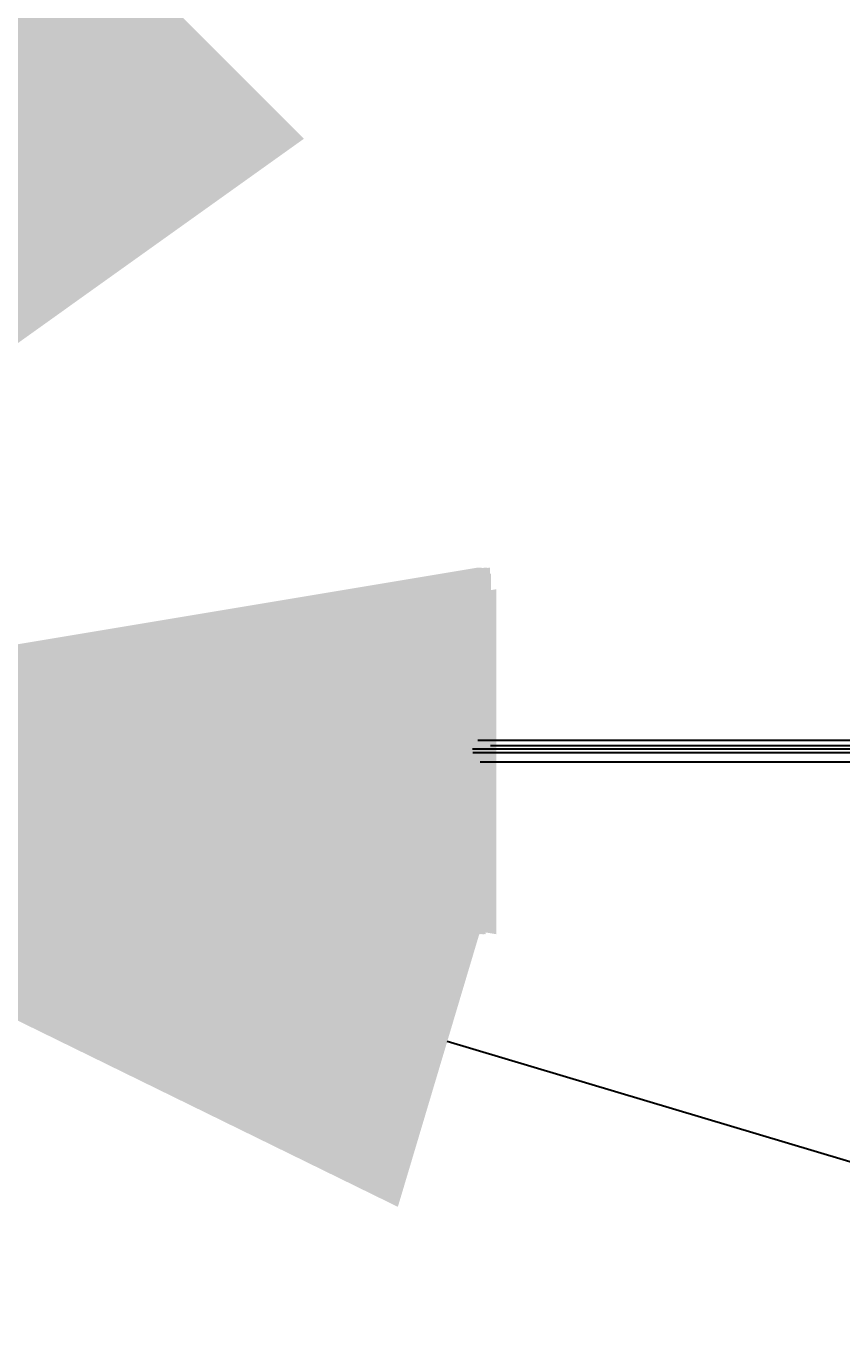
# Model space of a CAD drawing. Units: millimetres. Extents: x -22994 to 29398, y -19990 to 20176.
# Tile 133 of 135: x 5745 to 13629, y -5571 to 7102. Entities that reach past the tile are written whole.
import ezdxf

# ---------------------------------------------------------------- set-up
doc = ezdxf.new("R2010")
doc.units = ezdxf.units.MM
doc.header["$MEASUREMENT"] = 0
doc.layers.add('M-DIMS', color=2, linetype='Continuous', lineweight=18)
doc.styles.get("Standard").update_dxf_attribs({"font": 'arial.ttf'})
doc.dimstyles.get("Standard").update_dxf_attribs({"dimtxt": 0.18, "dimasz": 10000, "dimexe": 0.18, "dimexo": 0.0625, "dimgap": 0.09, "dimtad": 0, "dimtih": 1, "dimtoh": 1, "dimdec": 0, "dimzin": 0, "dimdsep": 46, "dimtxsty": 'Standard', "dimcen": 0.09, "dimadec": 0, "dimazin": 0, "dimtfac": 1, "dimtdec": 0, "dimtofl": 0, "dimtmove": 0, "dimatfit": 3, "dimfxl": 1, "dimtolj": 1, "dimtzin": 0, "dimlwd": 30, "dimarcsym": 0})

# ---------------------------------------------------------------- blocks, each defined once
blk = doc.blocks.new('*D2')
at = {"layer": 'Defpoints', "color": 0, "transparency": 16777216}
for p in [(7, 10), (291, 10), (291, -5)]:
    blk.add_point(p, dxfattribs=at)
at = {"layer": 'M-DIMS', "color": 0, "lineweight": -2, "transparency": 16777216}
for p, q in [((7, 10), (7, -5)), ((291, 10), (291, -5))]:
    blk.add_line(p, q, dxfattribs=at)
at = {"layer": 'M-DIMS', "color": 0, "lineweight": 30, "transparency": 16777216}
for p, q in [((-9993, -5), (-19993, -5)), ((10291, -5), (20291, -5))]:
    blk.add_line(p, q, dxfattribs=at)
at = {"layer": 'M-DIMS', "color": 0, "transparency": 16777216}
for points in [[(-9993, 1662), (-9993, -1672), (7, -5)], [(10291, 1662), (10291, -1672), (291, -5)]]:
    blk.add_solid(points, dxfattribs=at)
at = {"layer": 'M-DIMS', "color": 0, "transparency": 16777216, "insert": (149, -5), "char_height": 0.18, "attachment_point": 5}
blk.add_mtext('\\A1;284.2', dxfattribs=at)
blk = doc.blocks.new('*D3')
at = {"layer": 'Defpoints', "color": 0, "transparency": 16777216}
for p in [(96, 128), (110, 204), (110, 176)]:
    blk.add_point(p, dxfattribs=at)
at = {"layer": 'M-DIMS', "color": 0, "lineweight": 30, "transparency": 16777216}
for p, q in [((-9904, 204), (-19904, 204)), ((10110, 204), (20110, 204))]:
    blk.add_line(p, q, dxfattribs=at)
at = {"layer": 'M-DIMS', "color": 0, "lineweight": -2, "transparency": 16777216}
for p, q in [((96, 128), (96, 204)), ((110, 176), (110, 204))]:
    blk.add_line(p, q, dxfattribs=at)
at = {"layer": 'M-DIMS', "color": 0, "transparency": 16777216}
for points in [[(-9904, 1871), (-9904, -1463), (96, 204)], [(10110, 1871), (10110, -1463), (110, 204)]]:
    blk.add_solid(points, dxfattribs=at)
at = {"layer": 'M-DIMS', "color": 0, "transparency": 16777216, "insert": (103, 204), "char_height": 0.18, "attachment_point": 5}
blk.add_mtext('\\A1;14.432', dxfattribs=at)
blk = doc.blocks.new('*D4')
at = {"layer": 'Defpoints', "color": 0, "transparency": 16777216}
for p in [(110, 176), (116, 204), (116, 176)]:
    blk.add_point(p, dxfattribs=at)
at = {"layer": 'M-DIMS', "color": 0, "lineweight": 30, "transparency": 16777216}
for p, q in [((-9890, 204), (-19890, 204)), ((10116, 204), (20116, 204))]:
    blk.add_line(p, q, dxfattribs=at)
at = {"layer": 'M-DIMS', "color": 0, "lineweight": -2, "transparency": 16777216}
for p, q in [((110, 176), (110, 204)), ((116, 176), (116, 204))]:
    blk.add_line(p, q, dxfattribs=at)
at = {"layer": 'M-DIMS', "color": 0, "transparency": 16777216}
for points in [[(-9890, 1871), (-9890, -1463), (110, 204)], [(10116, 1871), (10116, -1463), (116, 204)]]:
    blk.add_solid(points, dxfattribs=at)
at = {"layer": 'M-DIMS', "color": 0, "transparency": 16777216, "insert": (113, 204), "char_height": 0.18, "attachment_point": 5}
blk.add_mtext('\\A1;6', dxfattribs=at)
blk = doc.blocks.new('*D5')
at = {"layer": 'Defpoints', "color": 0, "transparency": 16777216}
for p in [(116, 176), (181, 204), (181, 176)]:
    blk.add_point(p, dxfattribs=at)
at = {"layer": 'M-DIMS', "color": 0, "lineweight": 30, "transparency": 16777216}
for p, q in [((-9884, 204), (-19884, 204)), ((10181, 204), (20181, 204))]:
    blk.add_line(p, q, dxfattribs=at)
at = {"layer": 'M-DIMS', "color": 0, "lineweight": -2, "transparency": 16777216}
for p, q in [((116, 176), (116, 204)), ((181, 176), (181, 204))]:
    blk.add_line(p, q, dxfattribs=at)
at = {"layer": 'M-DIMS', "color": 0, "transparency": 16777216}
for points in [[(-9884, 1871), (-9884, -1463), (116, 204)], [(10181, 1871), (10181, -1463), (181, 204)]]:
    blk.add_solid(points, dxfattribs=at)
at = {"layer": 'M-DIMS', "color": 0, "transparency": 16777216, "insert": (149, 204), "char_height": 0.18, "attachment_point": 5}
blk.add_mtext('\\A1;65', dxfattribs=at)
blk = doc.blocks.new('*D6')
at = {"layer": 'Defpoints', "color": 0, "transparency": 16777216}
for p in [(181, 176), (187, 204), (187, 176)]:
    blk.add_point(p, dxfattribs=at)
at = {"layer": 'M-DIMS', "color": 0, "lineweight": 30, "transparency": 16777216}
for p, q in [((-9819, 204), (-19819, 204)), ((10187, 204), (20187, 204))]:
    blk.add_line(p, q, dxfattribs=at)
at = {"layer": 'M-DIMS', "color": 0, "lineweight": -2, "transparency": 16777216}
for p, q in [((181, 176), (181, 204)), ((187, 176), (187, 204))]:
    blk.add_line(p, q, dxfattribs=at)
at = {"layer": 'M-DIMS', "color": 0, "transparency": 16777216}
for points in [[(-9819, 1871), (-9819, -1463), (181, 204)], [(10187, 1871), (10187, -1463), (187, 204)]]:
    blk.add_solid(points, dxfattribs=at)
at = {"layer": 'M-DIMS', "color": 0, "transparency": 16777216, "insert": (184, 204), "char_height": 0.18, "attachment_point": 5}
blk.add_mtext('\\A1;6', dxfattribs=at)
blk = doc.blocks.new('*D7')
at = {"layer": 'Defpoints', "color": 0, "transparency": 16777216}
for p in [(187, 176), (202, 204), (202, 128)]:
    blk.add_point(p, dxfattribs=at)
at = {"layer": 'M-DIMS', "color": 0, "lineweight": 30, "transparency": 16777216}
for p, q in [((-9813, 204), (-19813, 204)), ((10202, 204), (20202, 204))]:
    blk.add_line(p, q, dxfattribs=at)
at = {"layer": 'M-DIMS', "color": 0, "lineweight": -2, "transparency": 16777216}
for p, q in [((187, 176), (187, 204)), ((202, 128), (202, 204))]:
    blk.add_line(p, q, dxfattribs=at)
at = {"layer": 'M-DIMS', "color": 0, "transparency": 16777216}
for points in [[(-9813, 1871), (-9813, -1463), (187, 204)], [(10202, 1871), (10202, -1463), (202, 204)]]:
    blk.add_solid(points, dxfattribs=at)
at = {"layer": 'M-DIMS', "color": 0, "transparency": 16777216, "insert": (194, 204), "char_height": 0.18, "attachment_point": 5}
blk.add_mtext('\\A1;14.432', dxfattribs=at)
blk = doc.blocks.new('*D8')
at = {"layer": 'Defpoints', "color": 0, "transparency": 16777216}
for p in [(202, 128), (228, 204), (228, 147)]:
    blk.add_point(p, dxfattribs=at)
at = {"layer": 'M-DIMS', "color": 0, "lineweight": 30, "transparency": 16777216}
for p, q in [((-9798, 204), (-19798, 204)), ((10228, 204), (20228, 204))]:
    blk.add_line(p, q, dxfattribs=at)
at = {"layer": 'M-DIMS', "color": 0, "lineweight": -2, "transparency": 16777216}
for p, q in [((202, 128), (202, 204)), ((228, 147), (228, 204))]:
    blk.add_line(p, q, dxfattribs=at)
at = {"layer": 'M-DIMS', "color": 0, "transparency": 16777216}
for points in [[(-9798, 1871), (-9798, -1463), (202, 204)], [(10228, 1871), (10228, -1463), (228, 204)]]:
    blk.add_solid(points, dxfattribs=at)
at = {"layer": 'M-DIMS', "color": 0, "transparency": 16777216, "insert": (215, 204), "char_height": 0.18, "attachment_point": 5}
blk.add_mtext('\\A1;25.95', dxfattribs=at)
blk = doc.blocks.new('*D10')
at = {"layer": 'Defpoints', "color": 0, "transparency": 16777216}
for p in [(126, 136), (133, 136), (133, -5)]:
    blk.add_point(p, dxfattribs=at)
at = {"layer": 'M-DIMS', "color": 0, "lineweight": -2, "transparency": 16777216}
for p, q in [((126, 136), (126, -5)), ((133, 136), (133, -5))]:
    blk.add_line(p, q, dxfattribs=at)
at = {"layer": 'M-DIMS', "color": 0, "lineweight": 30, "transparency": 16777216}
for p, q in [((-9874, -5), (-19874, -5)), ((10133, -5), (20133, -5))]:
    blk.add_line(p, q, dxfattribs=at)
at = {"layer": 'M-DIMS', "color": 0, "transparency": 16777216}
for points in [[(-9874, 1662), (-9874, -1672), (126, -5)], [(10133, 1662), (10133, -1672), (133, -5)]]:
    blk.add_solid(points, dxfattribs=at)
at = {"layer": 'M-DIMS', "color": 0, "transparency": 16777216, "insert": (129, -5), "char_height": 0.18, "attachment_point": 5}
blk.add_mtext('\\A1;7.696', dxfattribs=at)
blk = doc.blocks.new('*D11')
at = {"layer": 'Defpoints', "color": 0, "transparency": 16777216}
for p in [(133, 136), (136, 136), (136, -5)]:
    blk.add_point(p, dxfattribs=at)
at = {"layer": 'M-DIMS', "color": 0, "lineweight": -2, "transparency": 16777216}
for p, q in [((133, 136), (133, -5)), ((136, 136), (136, -5))]:
    blk.add_line(p, q, dxfattribs=at)
at = {"layer": 'M-DIMS', "color": 0, "lineweight": 30, "transparency": 16777216}
for p, q in [((-9867, -5), (-19867, -5)), ((10136, -5), (20136, -5))]:
    blk.add_line(p, q, dxfattribs=at)
at = {"layer": 'M-DIMS', "color": 0, "transparency": 16777216}
for points in [[(-9867, 1662), (-9867, -1672), (133, -5)], [(10136, 1662), (10136, -1672), (136, -5)]]:
    blk.add_solid(points, dxfattribs=at)
at = {"layer": 'M-DIMS', "color": 0, "transparency": 16777216, "insert": (134, -5), "char_height": 0.18, "attachment_point": 5}
blk.add_mtext('\\A1;2.304', dxfattribs=at)
blk = doc.blocks.new('*D12')
at = {"layer": 'Defpoints', "color": 0, "transparency": 16777216}
for p in [(136, 136), (146, 136), (146, -5)]:
    blk.add_point(p, dxfattribs=at)
at = {"layer": 'M-DIMS', "color": 0, "lineweight": -2, "transparency": 16777216}
for p, q in [((136, 136), (136, -5)), ((146, 136), (146, -5))]:
    blk.add_line(p, q, dxfattribs=at)
at = {"layer": 'M-DIMS', "color": 0, "lineweight": 30, "transparency": 16777216}
for p, q in [((-9864, -5), (-19864, -5)), ((10146, -5), (20146, -5))]:
    blk.add_line(p, q, dxfattribs=at)
at = {"layer": 'M-DIMS', "color": 0, "transparency": 16777216}
for points in [[(-9864, 1662), (-9864, -1672), (136, -5)], [(10146, 1662), (10146, -1672), (146, -5)]]:
    blk.add_solid(points, dxfattribs=at)
at = {"layer": 'M-DIMS', "color": 0, "transparency": 16777216, "insert": (141, -5), "char_height": 0.18, "attachment_point": 5}
blk.add_mtext('\\A1;10', dxfattribs=at)
blk = doc.blocks.new('*D13')
at = {"layer": 'Defpoints', "color": 0, "transparency": 16777216}
for p in [(146, 136), (156, 136), (156, -5)]:
    blk.add_point(p, dxfattribs=at)
at = {"layer": 'M-DIMS', "color": 0, "lineweight": -2, "transparency": 16777216}
for p, q in [((146, 136), (146, -5)), ((156, 136), (156, -5))]:
    blk.add_line(p, q, dxfattribs=at)
at = {"layer": 'M-DIMS', "color": 0, "lineweight": 30, "transparency": 16777216}
for p, q in [((-9854, -5), (-19854, -5)), ((10156, -5), (20156, -5))]:
    blk.add_line(p, q, dxfattribs=at)
at = {"layer": 'M-DIMS', "color": 0, "transparency": 16777216}
for points in [[(-9854, 1662), (-9854, -1672), (146, -5)], [(10156, 1662), (10156, -1672), (156, -5)]]:
    blk.add_solid(points, dxfattribs=at)
at = {"layer": 'M-DIMS', "color": 0, "transparency": 16777216, "insert": (151, -5), "char_height": 0.18, "attachment_point": 5}
blk.add_mtext('\\A1;10', dxfattribs=at)
blk = doc.blocks.new('*D14')
at = {"layer": 'Defpoints', "color": 0, "transparency": 16777216}
for p in [(156, 136), (166, 136), (166, -5)]:
    blk.add_point(p, dxfattribs=at)
at = {"layer": 'M-DIMS', "color": 0, "lineweight": -2, "transparency": 16777216}
for p, q in [((156, 136), (156, -5)), ((166, 136), (166, -5))]:
    blk.add_line(p, q, dxfattribs=at)
at = {"layer": 'M-DIMS', "color": 0, "lineweight": 30, "transparency": 16777216}
for p, q in [((-9844, -5), (-19844, -5)), ((10166, -5), (20166, -5))]:
    blk.add_line(p, q, dxfattribs=at)
at = {"layer": 'M-DIMS', "color": 0, "transparency": 16777216}
for points in [[(-9844, 1662), (-9844, -1672), (156, -5)], [(10166, 1662), (10166, -1672), (166, -5)]]:
    blk.add_solid(points, dxfattribs=at)
at = {"layer": 'M-DIMS', "color": 0, "transparency": 16777216, "insert": (161, -5), "char_height": 0.18, "attachment_point": 5}
blk.add_mtext('\\A1;10', dxfattribs=at)
blk = doc.blocks.new('*D16')
at = {"layer": 'Defpoints', "color": 0, "transparency": 16777216}
for p in [(120, 204), (110, 48), (120, 48)]:
    blk.add_point(p, dxfattribs=at)
at = {"layer": 'M-DIMS', "color": 0, "lineweight": 30, "transparency": 16777216}
for p, q in [((-9890, 204), (-19890, 204)), ((10120, 204), (20120, 204))]:
    blk.add_line(p, q, dxfattribs=at)
at = {"layer": 'M-DIMS', "color": 0, "lineweight": -2, "transparency": 16777216}
for p, q in [((110, 48), (110, 204)), ((120, 48), (120, 204))]:
    blk.add_line(p, q, dxfattribs=at)
at = {"layer": 'M-DIMS', "color": 0, "transparency": 16777216}
for points in [[(-9890, 1871), (-9890, -1463), (110, 204)], [(10120, 1871), (10120, -1463), (120, 204)]]:
    blk.add_solid(points, dxfattribs=at)
at = {"layer": 'M-DIMS', "color": 0, "transparency": 16777216, "insert": (115, 204), "char_height": 0.18, "attachment_point": 5}
blk.add_mtext('\\A1;9.704', dxfattribs=at)
blk = doc.blocks.new('*D17')
at = {"layer": 'Defpoints', "color": 0, "transparency": 16777216}
for p in [(126, 204), (120, 48), (126, 48)]:
    blk.add_point(p, dxfattribs=at)
at = {"layer": 'M-DIMS', "color": 0, "lineweight": 30, "transparency": 16777216}
for p, q in [((-9880, 204), (-19880, 204)), ((10126, 204), (20126, 204))]:
    blk.add_line(p, q, dxfattribs=at)
at = {"layer": 'M-DIMS', "color": 0, "lineweight": -2, "transparency": 16777216}
for p, q in [((120, 48), (120, 204)), ((126, 48), (126, 204))]:
    blk.add_line(p, q, dxfattribs=at)
at = {"layer": 'M-DIMS', "color": 0, "transparency": 16777216}
for points in [[(-9880, 1871), (-9880, -1463), (120, 204)], [(10126, 1871), (10126, -1463), (126, 204)]]:
    blk.add_solid(points, dxfattribs=at)
at = {"layer": 'M-DIMS', "color": 0, "transparency": 16777216, "insert": (123, 204), "char_height": 0.18, "attachment_point": 5}
blk.add_mtext('\\A1;6', dxfattribs=at)
blk = doc.blocks.new('*D18')
at = {"layer": 'Defpoints', "color": 0, "transparency": 16777216}
for p in [(132, 204), (126, 48), (132, 48)]:
    blk.add_point(p, dxfattribs=at)
at = {"layer": 'M-DIMS', "color": 0, "lineweight": 30, "transparency": 16777216}
for p, q in [((-9874, 204), (-19874, 204)), ((10132, 204), (20132, 204))]:
    blk.add_line(p, q, dxfattribs=at)
at = {"layer": 'M-DIMS', "color": 0, "lineweight": -2, "transparency": 16777216}
for p, q in [((126, 48), (126, 204)), ((132, 48), (132, 204))]:
    blk.add_line(p, q, dxfattribs=at)
at = {"layer": 'M-DIMS', "color": 0, "transparency": 16777216}
for points in [[(-9874, 1871), (-9874, -1463), (126, 204)], [(10132, 1871), (10132, -1463), (132, 204)]]:
    blk.add_solid(points, dxfattribs=at)
at = {"layer": 'M-DIMS', "color": 0, "transparency": 16777216, "insert": (129, 204), "char_height": 0.18, "attachment_point": 5}
blk.add_mtext('\\A1;6', dxfattribs=at)
blk = doc.blocks.new('*D19')
at = {"layer": 'Defpoints', "color": 0, "transparency": 16777216}
for p in [(138, 204), (132, 48), (138, 48)]:
    blk.add_point(p, dxfattribs=at)
at = {"layer": 'M-DIMS', "color": 0, "lineweight": 30, "transparency": 16777216}
for p, q in [((-9868, 204), (-19868, 204)), ((10138, 204), (20138, 204))]:
    blk.add_line(p, q, dxfattribs=at)
at = {"layer": 'M-DIMS', "color": 0, "lineweight": -2, "transparency": 16777216}
for p, q in [((132, 48), (132, 204)), ((138, 48), (138, 204))]:
    blk.add_line(p, q, dxfattribs=at)
at = {"layer": 'M-DIMS', "color": 0, "transparency": 16777216}
for points in [[(-9868, 1871), (-9868, -1463), (132, 204)], [(10138, 1871), (10138, -1463), (138, 204)]]:
    blk.add_solid(points, dxfattribs=at)
at = {"layer": 'M-DIMS', "color": 0, "transparency": 16777216, "insert": (135, 204), "char_height": 0.18, "attachment_point": 5}
blk.add_mtext('\\A1;6', dxfattribs=at)
blk = doc.blocks.new('*D20')
at = {"layer": 'Defpoints', "color": 0, "transparency": 16777216}
for p in [(144, 204), (138, 48), (144, 48)]:
    blk.add_point(p, dxfattribs=at)
at = {"layer": 'M-DIMS', "color": 0, "lineweight": 30, "transparency": 16777216}
for p, q in [((-9862, 204), (-19862, 204)), ((10144, 204), (20144, 204))]:
    blk.add_line(p, q, dxfattribs=at)
at = {"layer": 'M-DIMS', "color": 0, "lineweight": -2, "transparency": 16777216}
for p, q in [((138, 48), (138, 204)), ((144, 48), (144, 204))]:
    blk.add_line(p, q, dxfattribs=at)
at = {"layer": 'M-DIMS', "color": 0, "transparency": 16777216}
for points in [[(-9862, 1871), (-9862, -1463), (138, 204)], [(10144, 1871), (10144, -1463), (144, 204)]]:
    blk.add_solid(points, dxfattribs=at)
at = {"layer": 'M-DIMS', "color": 0, "transparency": 16777216, "insert": (141, 204), "char_height": 0.18, "attachment_point": 5}
blk.add_mtext('\\A1;6', dxfattribs=at)
blk = doc.blocks.new('*D21')
at = {"layer": 'Defpoints', "color": 0, "transparency": 16777216}
for p in [(149, 204), (144, 48), (149, 48)]:
    blk.add_point(p, dxfattribs=at)
at = {"layer": 'M-DIMS', "color": 0, "lineweight": 30, "transparency": 16777216}
for p, q in [((-9856, 204), (-19856, 204)), ((10149, 204), (20149, 204))]:
    blk.add_line(p, q, dxfattribs=at)
at = {"layer": 'M-DIMS', "color": 0, "lineweight": -2, "transparency": 16777216}
for p, q in [((144, 48), (144, 204)), ((149, 48), (149, 204))]:
    blk.add_line(p, q, dxfattribs=at)
at = {"layer": 'M-DIMS', "color": 0, "transparency": 16777216}
for points in [[(-9856, 1871), (-9856, -1463), (144, 204)], [(10149, 1871), (10149, -1463), (149, 204)]]:
    blk.add_solid(points, dxfattribs=at)
at = {"layer": 'M-DIMS', "color": 0, "transparency": 16777216, "insert": (147, 204), "char_height": 0.18, "attachment_point": 5}
blk.add_mtext('\\A1;4.945', dxfattribs=at)
blk = doc.blocks.new('*D22')
at = {"layer": 'Defpoints', "color": 0, "transparency": 16777216}
for p in [(149, 31), (155, 31), (155, -5)]:
    blk.add_point(p, dxfattribs=at)
at = {"layer": 'M-DIMS', "color": 0, "lineweight": -2, "transparency": 16777216}
for p, q in [((149, 31), (149, -5)), ((155, 31), (155, -5))]:
    blk.add_line(p, q, dxfattribs=at)
at = {"layer": 'M-DIMS', "color": 0, "lineweight": 30, "transparency": 16777216}
for p, q in [((-9851, -5), (-19851, -5)), ((10155, -5), (20155, -5))]:
    blk.add_line(p, q, dxfattribs=at)
at = {"layer": 'M-DIMS', "color": 0, "transparency": 16777216}
for points in [[(-9851, 1662), (-9851, -1672), (149, -5)], [(10155, 1662), (10155, -1672), (155, -5)]]:
    blk.add_solid(points, dxfattribs=at)
at = {"layer": 'M-DIMS', "color": 0, "transparency": 16777216, "insert": (152, -5), "char_height": 0.18, "attachment_point": 5}
blk.add_mtext('\\A1;6', dxfattribs=at)
blk = doc.blocks.new('*D23')
at = {"layer": 'Defpoints', "color": 0, "transparency": 16777216}
for p in [(155, 31), (161, 31), (161, -5)]:
    blk.add_point(p, dxfattribs=at)
at = {"layer": 'M-DIMS', "color": 0, "lineweight": -2, "transparency": 16777216}
for p, q in [((155, 31), (155, -5)), ((161, 31), (161, -5))]:
    blk.add_line(p, q, dxfattribs=at)
at = {"layer": 'M-DIMS', "color": 0, "lineweight": 30, "transparency": 16777216}
for p, q in [((-9845, -5), (-19845, -5)), ((10161, -5), (20161, -5))]:
    blk.add_line(p, q, dxfattribs=at)
at = {"layer": 'M-DIMS', "color": 0, "transparency": 16777216}
for points in [[(-9845, 1662), (-9845, -1672), (155, -5)], [(10161, 1662), (10161, -1672), (161, -5)]]:
    blk.add_solid(points, dxfattribs=at)
at = {"layer": 'M-DIMS', "color": 0, "transparency": 16777216, "insert": (158, -5), "char_height": 0.18, "attachment_point": 5}
blk.add_mtext('\\A1;6', dxfattribs=at)
blk = doc.blocks.new('*D24')
at = {"layer": 'Defpoints', "color": 0, "transparency": 16777216}
for p in [(161, 31), (166, 31), (166, -5)]:
    blk.add_point(p, dxfattribs=at)
at = {"layer": 'M-DIMS', "color": 0, "lineweight": -2, "transparency": 16777216}
for p, q in [((161, 31), (161, -5)), ((166, 31), (166, -5))]:
    blk.add_line(p, q, dxfattribs=at)
at = {"layer": 'M-DIMS', "color": 0, "lineweight": 30, "transparency": 16777216}
for p, q in [((-9839, -5), (-19839, -5)), ((10166, -5), (20166, -5))]:
    blk.add_line(p, q, dxfattribs=at)
at = {"layer": 'M-DIMS', "color": 0, "transparency": 16777216}
for points in [[(-9839, 1662), (-9839, -1672), (161, -5)], [(10166, 1662), (10166, -1672), (166, -5)]]:
    blk.add_solid(points, dxfattribs=at)
at = {"layer": 'M-DIMS', "color": 0, "transparency": 16777216, "insert": (164, -5), "char_height": 0.18, "attachment_point": 5}
blk.add_mtext('\\A1;5.323', dxfattribs=at)
blk = doc.blocks.new('*D25')
at = {"layer": 'Defpoints', "color": 0, "transparency": 16777216}
for p in [(166, 31), (172, 31), (172, -5)]:
    blk.add_point(p, dxfattribs=at)
at = {"layer": 'M-DIMS', "color": 0, "lineweight": -2, "transparency": 16777216}
for p, q in [((166, 31), (166, -5)), ((172, 31), (172, -5))]:
    blk.add_line(p, q, dxfattribs=at)
at = {"layer": 'M-DIMS', "color": 0, "lineweight": 30, "transparency": 16777216}
for p, q in [((-9834, -5), (-19834, -5)), ((10172, -5), (20172, -5))]:
    blk.add_line(p, q, dxfattribs=at)
at = {"layer": 'M-DIMS', "color": 0, "transparency": 16777216}
for points in [[(-9834, 1662), (-9834, -1672), (166, -5)], [(10172, 1662), (10172, -1672), (172, -5)]]:
    blk.add_solid(points, dxfattribs=at)
at = {"layer": 'M-DIMS', "color": 0, "transparency": 16777216, "insert": (169, -5), "char_height": 0.18, "attachment_point": 5}
blk.add_mtext('\\A1;6', dxfattribs=at)
blk = doc.blocks.new('*D26')
at = {"layer": 'Defpoints', "color": 0, "transparency": 16777216}
for p in [(172, 31), (178, 31), (178, -5)]:
    blk.add_point(p, dxfattribs=at)
at = {"layer": 'M-DIMS', "color": 0, "lineweight": -2, "transparency": 16777216}
for p, q in [((172, 31), (172, -5)), ((178, 31), (178, -5))]:
    blk.add_line(p, q, dxfattribs=at)
at = {"layer": 'M-DIMS', "color": 0, "lineweight": 30, "transparency": 16777216}
for p, q in [((-9828, -5), (-19828, -5)), ((10178, -5), (20178, -5))]:
    blk.add_line(p, q, dxfattribs=at)
at = {"layer": 'M-DIMS', "color": 0, "transparency": 16777216}
for points in [[(-9828, 1662), (-9828, -1672), (172, -5)], [(10178, 1662), (10178, -1672), (178, -5)]]:
    blk.add_solid(points, dxfattribs=at)
at = {"layer": 'M-DIMS', "color": 0, "transparency": 16777216, "insert": (175, -5), "char_height": 0.18, "attachment_point": 5}
blk.add_mtext('\\A1;6', dxfattribs=at)
blk = doc.blocks.new('*D27')
at = {"layer": 'Defpoints', "color": 0, "transparency": 16777216}
for p in [(178, 31), (188, 31), (188, -5)]:
    blk.add_point(p, dxfattribs=at)
at = {"layer": 'M-DIMS', "color": 0, "lineweight": -2, "transparency": 16777216}
for p, q in [((178, 31), (178, -5)), ((188, 31), (188, -5))]:
    blk.add_line(p, q, dxfattribs=at)
at = {"layer": 'M-DIMS', "color": 0, "lineweight": 30, "transparency": 16777216}
for p, q in [((-9822, -5), (-19822, -5)), ((10188, -5), (20188, -5))]:
    blk.add_line(p, q, dxfattribs=at)
at = {"layer": 'M-DIMS', "color": 0, "transparency": 16777216}
for points in [[(-9822, 1662), (-9822, -1672), (178, -5)], [(10188, 1662), (10188, -1672), (188, -5)]]:
    blk.add_solid(points, dxfattribs=at)
at = {"layer": 'M-DIMS', "color": 0, "transparency": 16777216, "insert": (183, -5), "char_height": 0.18, "attachment_point": 5}
blk.add_mtext('\\A1;9.679', dxfattribs=at)
blk = doc.blocks.new('*D29')
at = {"layer": 'Defpoints', "color": 0, "transparency": 16777216}
for p in [(37, 80), (64, 80)]:
    blk.add_point(p, dxfattribs=at)
at = {"layer": 'M-DIMS', "color": 0, "lineweight": -2, "transparency": 16777216}
for q in [(51, 80), (50, 80)]:
    blk.add_line((50, 80), q, dxfattribs=at)
at = {"layer": 'M-DIMS', "color": 0, "lineweight": 30, "transparency": 16777216}
blk.add_line((20064, 80), (10064, 80), dxfattribs=at)
at = {"layer": 'M-DIMS', "color": 0, "transparency": 16777216}
blk.add_solid([(10064, 1747), (10064, -1587), (64, 80)], dxfattribs=at)
at = {"layer": 'M-DIMS', "color": 0, "transparency": 16777216, "insert": (20065, 80), "char_height": 0.18, "attachment_point": 5}
blk.add_mtext('\\A1;∅27.23', dxfattribs=at)
blk = doc.blocks.new('*D30')
at = {"layer": 'Defpoints', "color": 0, "transparency": 16777216}
for p in [(216, 147), (239, 147)]:
    blk.add_point(p, dxfattribs=at)
at = {"layer": 'M-DIMS', "color": 0, "lineweight": -2, "transparency": 16777216}
blk.add_line((228, 147), (228, 147), dxfattribs=at)
blk.add_line((228, 147), (228, 147), dxfattribs=at)
at = {"layer": 'M-DIMS', "color": 0, "lineweight": 30, "transparency": 16777216}
blk.add_line((20239, 147), (10239, 147), dxfattribs=at)
at = {"layer": 'M-DIMS', "color": 0, "transparency": 16777216}
blk.add_solid([(10239, 1814), (10239, -1520), (239, 147)], dxfattribs=at)
at = {"layer": 'M-DIMS', "color": 0, "transparency": 16777216, "insert": (20240, 147), "char_height": 0.18, "attachment_point": 5}
blk.add_mtext('\\A1;∅22.667', dxfattribs=at)
blk = doc.blocks.new('*D31')
at = {"layer": 'Defpoints', "color": 0, "transparency": 16777216}
for p in [(223, 147), (232, 147)]:
    blk.add_point(p, dxfattribs=at)
at = {"layer": 'M-DIMS', "color": 0, "lineweight": -2, "transparency": 16777216}
blk.add_line((228, 147), (228, 147), dxfattribs=at)
blk.add_line((228, 147), (228, 147), dxfattribs=at)
at = {"layer": 'M-DIMS', "color": 0, "lineweight": 30, "transparency": 16777216}
blk.add_line((20232, 149), (10232, 148), dxfattribs=at)
at = {"layer": 'M-DIMS', "color": 0, "transparency": 16777216}
blk.add_solid([(10232, 1814), (10232, -1519), (232, 147)], dxfattribs=at)
at = {"layer": 'M-DIMS', "color": 0, "transparency": 16777216, "insert": (20233, 149), "char_height": 0.18, "attachment_point": 5}
blk.add_mtext('\\A1;∅8.969', dxfattribs=at)
blk = doc.blocks.new('*D33')
at = {"layer": 'Defpoints', "color": 0, "transparency": 16777216}
for p in [(230, 154), (233, 153)]:
    blk.add_point(p, dxfattribs=at)
at = {"layer": 'M-DIMS', "color": 0, "lineweight": -2, "transparency": 16777216}
for p in [(229, 154), (230, 154)]:
    blk.add_line(p, (230, 154), dxfattribs=at)
at = {"layer": 'M-DIMS', "color": 0, "lineweight": 30, "transparency": 16777216}
for p, q in [((19396, -5571), (9815, -2709)), ((29396, -5571), (19396, -5571))]:
    blk.add_line(p, q, dxfattribs=at)
at = {"layer": 'M-DIMS', "color": 0, "transparency": 16777216}
blk.add_solid([(10292, -1112), (9338, -4306), (233, 153)], dxfattribs=at)
at = {"layer": 'M-DIMS', "color": 0, "transparency": 16777216, "insert": (29397, -5571), "char_height": 0.18, "attachment_point": 5}
blk.add_mtext('\\A1;6X R3.586', dxfattribs=at)
blk = doc.blocks.new('*D34')
at = {"layer": 'Defpoints', "color": 0, "transparency": 16777216}
for p in [(177, 121), (179, 123)]:
    blk.add_point(p, dxfattribs=at)
at = {"layer": 'M-DIMS', "color": 0, "lineweight": 30, "transparency": 16777216}
for p, q in [((14322, 14263), (7251, 7193)), ((24322, 14263), (14322, 14263))]:
    blk.add_line(p, q, dxfattribs=at)
at = {"layer": 'M-DIMS', "color": 0, "lineweight": -2, "transparency": 16777216}
blk.add_line((177, 121), (177, 121), dxfattribs=at)
blk.add_line((177, 121), (177, 121), dxfattribs=at)
at = {"layer": 'M-DIMS', "color": 0, "transparency": 16777216}
blk.add_solid([(6072, 8372), (8429, 6014), (179, 123)], dxfattribs=at)
at = {"layer": 'M-DIMS', "color": 0, "transparency": 16777216, "insert": (24323, 14263), "char_height": 0.18, "attachment_point": 5}
blk.add_mtext('\\A1;6X R2.5', dxfattribs=at)
blk = doc.blocks.new('*D36')
at = {"layer": 'Defpoints', "color": 0, "transparency": 16777216}
for p in [(46, 31), (46, 27)]:
    blk.add_point(p, dxfattribs=at)
at = {"layer": 'M-DIMS', "color": 0, "lineweight": 30, "transparency": 16777216}
for p, q in [((57, 20031), (52, 10031)), ((10057, 20031), (57, 20031))]:
    blk.add_line(p, q, dxfattribs=at)
at = {"layer": 'M-DIMS', "color": 0, "lineweight": -2, "transparency": 16777216}
blk.add_line((46, 29), (46, 29), dxfattribs=at)
blk.add_line((46, 29), (46, 29), dxfattribs=at)
at = {"layer": 'M-DIMS', "color": 0, "transparency": 16777216}
blk.add_solid([(-1615, 10032), (1718, 10030), (46, 31)], dxfattribs=at)
at = {"layer": 'M-DIMS', "color": 0, "transparency": 16777216, "insert": (10058, 20031), "char_height": 0.18, "attachment_point": 5}
blk.add_mtext('\\A1;∅4.71', dxfattribs=at)
blk = doc.blocks.new('*D37')
at = {"layer": 'Defpoints', "color": 0, "transparency": 16777216}
for p in [(55, 119), (59, 119)]:
    blk.add_point(p, dxfattribs=at)
at = {"layer": 'M-DIMS', "color": 0, "lineweight": -2, "transparency": 16777216}
blk.add_line((57, 119), (57, 119), dxfattribs=at)
blk.add_line((57, 119), (57, 119), dxfattribs=at)
at = {"layer": 'M-DIMS', "color": 0, "lineweight": 30, "transparency": 16777216}
blk.add_line((20059, 116), (10059, 117), dxfattribs=at)
at = {"layer": 'M-DIMS', "color": 0, "transparency": 16777216}
blk.add_solid([(10060, 1784), (10059, -1549), (59, 119)], dxfattribs=at)
at = {"layer": 'M-DIMS', "color": 0, "transparency": 16777216, "insert": (20060, 116), "char_height": 0.18, "attachment_point": 5}
blk.add_mtext('\\A1;∅4.659', dxfattribs=at)

msp = doc.modelspace()

# ---------------------------------------------------------------- dimensions: what is measured, and where the dimension line sits
at = {"layer": 'M-DIMS'}
for p1, p2, override, picture, middle in [((46.3875, 26.5934), (46.39, 31.3035), {"dimdec": 2, "dimlfac": 1, "dimrnd": 0, "dimzin": 0, "dimdsep": 46, "dimlunit": 2}, '*D36', (10057.5542, 20031.3006)), ((216.3148, 146.7291), (238.9821, 146.73), {"dimdec": 3, "dimlfac": 1, "dimrnd": 0, "dimzin": 0, "dimdsep": 46, "dimlunit": 2}, '*D30', (20238.9821, 147.4959)), ((223.1641, 146.7291), (232.1328, 146.73), {"dimdec": 3, "dimlfac": 1, "dimrnd": 0, "dimzin": 0, "dimdsep": 46, "dimlunit": 2}, '*D31', (20232.1327, 148.6656))]:
    dim = msp.add_diameter_dim_2p(p1=p1, p2=p2, dimstyle='Standard', override=override, dxfattribs=at)
    dim.commit()
    dim.dimension.update_dxf_attribs({"geometry": picture, "text_midpoint": middle, "dimtype": 163})
for center, mpoint, override, picture, middle in [((176.8123, 121.1277), (178.5802, 122.8952), {"dimdec": 1, "dimlfac": 1, "dimrnd": 0, "dimzin": 0, "dimdsep": 46, "dimlunit": 2}, '*D34', (24322.9703, 14263.3108)), ((229.5613, 154.3773), (232.9972, 153.3509), {"dimdec": 3, "dimlfac": 1, "dimrnd": 0, "dimzin": 0, "dimdsep": 46, "dimlunit": 2}, '*D33', (29397.0125, -5570.8378))]:
    dim = msp.add_radius_dim(center=center, mpoint=mpoint, text='6X <>', dimstyle='Standard', override=override, dxfattribs=at)
    dim.commit()
    dim.dimension.update_dxf_attribs({"geometry": picture, "text_midpoint": middle})
for base, p1, p2, override, picture, middle in [((110.2647, 204.1654), (95.8327, 127.967), (110.2647, 176.3662), {"dimdec": 3, "dimlfac": 1, "dimrnd": 0, "dimzin": 0, "dimdsep": 46, "dimlunit": 2}, '*D3', (103.0487, 204.1654)), ((116.2647, 204.1654), (110.2647, 176.3662), (116.2647, 176.3662), {"dimdec": 0, "dimlfac": 1, "dimrnd": 0, "dimzin": 0, "dimdsep": 46, "dimlunit": 2}, '*D4', (113.2647, 204.1654)), ((120.1702, 204.1654), (110.4658, 48.0349), (120.1702, 48.0349), {"dimdec": 3, "dimlfac": 1, "dimrnd": 0, "dimzin": 0, "dimdsep": 46, "dimlunit": 2}, '*D16', (115.318, 204.1654)), ((181.2647, 204.1654), (116.2647, 176.3662), (181.2647, 176.3662), {"dimdec": 0, "dimlfac": 1, "dimrnd": 0, "dimzin": 0, "dimdsep": 46, "dimlunit": 2}, '*D5', (148.7647, 204.1654)), ((126.1702, 204.1654), (120.1702, 48.0349), (126.1702, 48.0349), {"dimdec": 0, "dimlfac": 1, "dimrnd": 0, "dimzin": 0, "dimdsep": 46, "dimlunit": 2}, '*D17', (123.1702, 204.1654)), ((132.1702, 204.1654), (126.1702, 48.0349), (132.1702, 48.0349), {"dimdec": 0, "dimlfac": 1, "dimrnd": 0, "dimzin": 0, "dimdsep": 46, "dimlunit": 2}, '*D18', (129.1702, 204.1654)), ((138.1702, 204.1654), (132.1702, 48.0349), (138.1702, 48.0349), {"dimdec": 0, "dimlfac": 1, "dimrnd": 0, "dimzin": 0, "dimdsep": 46, "dimlunit": 2}, '*D19', (135.1702, 204.1654)), ((144.1702, 204.1654), (138.1702, 48.0349), (144.1702, 48.0349), {"dimdec": 0, "dimlfac": 1, "dimrnd": 0, "dimzin": 0, "dimdsep": 46, "dimlunit": 2}, '*D20', (141.1702, 204.1654)), ((149.11567, 204.16539), (144.17023, 48.03494), (149.11567, 48.03494), {"dimdec": 3, "dimlfac": 1, "dimrnd": 0, "dimzin": 0, "dimdsep": 46, "dimlunit": 2}, '*D21', (146.64295, 204.16539)), ((187.2647, 204.1654), (181.2647, 176.3662), (187.2647, 176.3662), {"dimdec": 0, "dimlfac": 1, "dimrnd": 0, "dimzin": 0, "dimdsep": 46, "dimlunit": 2}, '*D6', (184.2647, 204.1654)), ((201.6967, 204.1654), (187.2647, 176.3662), (201.6967, 127.967), {"dimdec": 3, "dimlfac": 1, "dimrnd": 0, "dimzin": 0, "dimdsep": 46, "dimlunit": 2}, '*D7', (194.4807, 204.1654)), ((227.6485, 204.1654), (201.6967, 127.967), (227.6485, 146.7296), {"dimdec": 2, "dimlfac": 1, "dimrnd": 0, "dimzin": 0, "dimdsep": 46, "dimlunit": 2}, '*D8', (214.6726, 204.1654)), ((290.852, -5.0787), (6.6773, 10.2713), (290.852, 10.2713), {"dimdec": 1, "dimlfac": 1, "dimrnd": 0, "dimzin": 0, "dimdsep": 46, "dimlunit": 2}, '*D2', (148.7647, -5.0787)), ((133.3459, -5.0787), (125.6498, 136.0713), (133.3459, 136.0713), {"dimdec": 3, "dimlfac": 1, "dimrnd": 0, "dimzin": 0, "dimdsep": 46, "dimlunit": 2}, '*D10', (129.4978, -5.0787)), ((135.6498, -5.0787), (133.3459, 136.0713), (135.6498, 136.0713), {"dimdec": 3, "dimlfac": 1, "dimrnd": 0, "dimzin": 0, "dimdsep": 46, "dimlunit": 2}, '*D11', (134.4978, -5.0787)), ((145.6498, -5.0787), (135.6498, 136.0713), (145.6498, 136.0713), {"dimdec": 0, "dimlfac": 1, "dimrnd": 0, "dimzin": 0, "dimdsep": 46, "dimlunit": 2}, '*D12', (140.6498, -5.0787)), ((155.6498, -5.0787), (145.6498, 136.0713), (155.6498, 136.0713), {"dimdec": 0, "dimlfac": 1, "dimrnd": 0, "dimzin": 0, "dimdsep": 46, "dimlunit": 2}, '*D13', (150.6498, -5.0787)), ((155.1157, -5.0787), (149.1157, 30.9895), (155.1157, 30.9895), {"dimdec": 0, "dimlfac": 1, "dimrnd": 0, "dimzin": 0, "dimdsep": 46, "dimlunit": 2}, '*D22', (152.1157, -5.0787)), ((161.1157, -5.0787), (155.1157, 30.9895), (161.1157, 30.9895), {"dimdec": 0, "dimlfac": 1, "dimrnd": 0, "dimzin": 0, "dimdsep": 46, "dimlunit": 2}, '*D23', (158.1157, -5.0787)), ((165.6498, -5.0787), (155.6498, 136.0713), (165.6498, 136.0713), {"dimdec": 0, "dimlfac": 1, "dimrnd": 0, "dimzin": 0, "dimdsep": 46, "dimlunit": 2}, '*D14', (160.6498, -5.0787)), ((166.4387, -5.0787), (161.1157, 30.9895), (166.4387, 30.9895), {"dimdec": 3, "dimlfac": 1, "dimrnd": 0, "dimzin": 0, "dimdsep": 46, "dimlunit": 2}, '*D24', (163.7772, -5.0787)), ((172.4387, -5.0787), (166.4387, 30.9895), (172.4387, 30.9895), {"dimdec": 0, "dimlfac": 1, "dimrnd": 0, "dimzin": 0, "dimdsep": 46, "dimlunit": 2}, '*D25', (169.4387, -5.0787)), ((178.4387, -5.0787), (172.4387, 30.9895), (178.4387, 30.9895), {"dimdec": 0, "dimlfac": 1, "dimrnd": 0, "dimzin": 0, "dimdsep": 46, "dimlunit": 2}, '*D26', (175.4387, -5.0787)), ((188.1175, -5.0787), (178.4387, 30.9895), (188.1175, 30.9895), {"dimdec": 3, "dimlfac": 1, "dimrnd": 0, "dimzin": 0, "dimdsep": 46, "dimlunit": 2}, '*D27', (183.2781, -5.0787))]:
    dim = msp.add_linear_dim(base=base, p1=p1, p2=p2, dimstyle='Standard', override=override, dxfattribs=at)
    dim.commit()
    dim.dimension.update_dxf_attribs({"geometry": picture, "text_midpoint": middle})
for p1, p2, override, picture, middle in [((54.8343, 118.6145), (59.4936, 118.614), {"dimdec": 3, "dimlfac": 1, "dimrnd": 0, "dimzin": 0, "dimdsep": 46, "dimlunit": 2}, '*D37', (20059.4934, 116.2531)), ((36.8006, 80.045), (64.0296, 80.045), {"dimdec": 2, "dimlfac": 1, "dimrnd": 0, "dimzin": 0, "dimdsep": 46, "dimlunit": 2}, '*D29', (20064.0296, 80.0303))]:
    dim = msp.add_diameter_dim_2p(p1=p1, p2=p2, dimstyle='Standard', override=override, dxfattribs=at)
    dim.commit()
    dim.dimension.update_dxf_attribs({"geometry": picture, "text_midpoint": middle})

doc.saveas('drawing.dxf')
